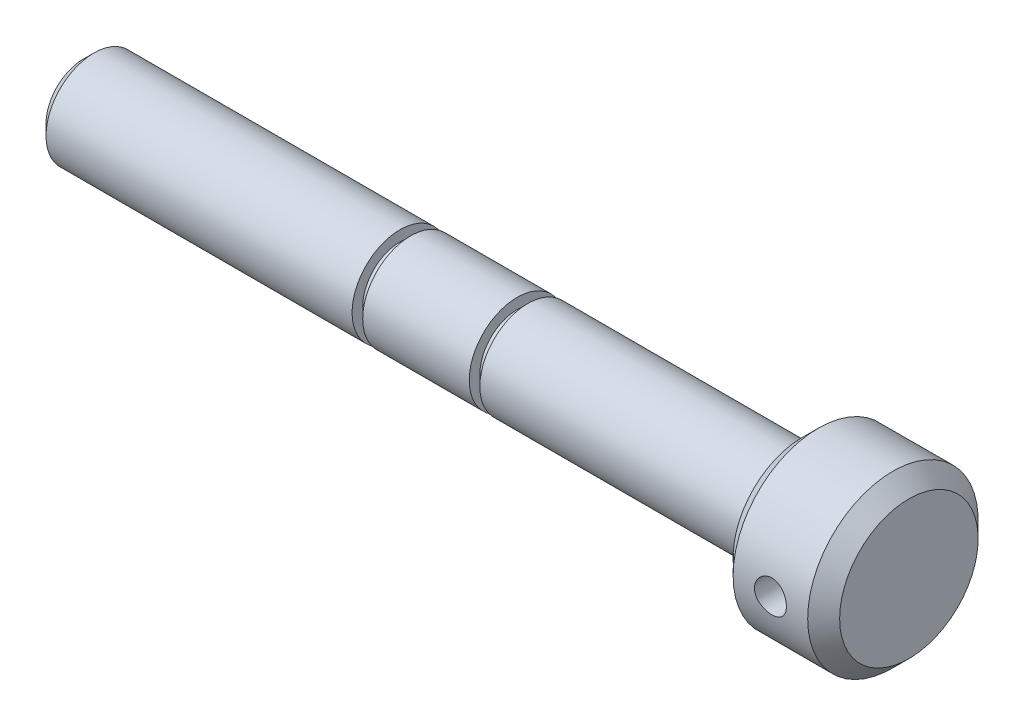
ISO-10303-21;
HEADER;
FILE_DESCRIPTION(('STEP AP214'),'2;1');
FILE_NAME('part.step','',(''),(''),'','','');
FILE_SCHEMA(('AUTOMOTIVE_DESIGN { 1 0 10303 214 1 1 1 1 }'));
ENDSEC;
DATA;
#1=APPLICATION_CONTEXT('core data for automotive mechanical design processes');
#2=APPLICATION_PROTOCOL_DEFINITION('international standard','automotive_design',2000,#1);
#3=PRODUCT_CONTEXT('',#1,'mechanical');
#4=PRODUCT('Part','Part','',(#3));
#5=PRODUCT_RELATED_PRODUCT_CATEGORY('part','',(#4));
#6=PRODUCT_DEFINITION_FORMATION('','',#4);
#7=PRODUCT_DEFINITION_CONTEXT('part definition',#1,'design');
#8=PRODUCT_DEFINITION('design','',#6,#7);
#9=PRODUCT_DEFINITION_SHAPE('','',#8);
#10=(LENGTH_UNIT() NAMED_UNIT(*) SI_UNIT(.MILLI.,.METRE.));
#11=(NAMED_UNIT(*) PLANE_ANGLE_UNIT() SI_UNIT($,.RADIAN.));
#12=(NAMED_UNIT(*) SI_UNIT($,.STERADIAN.) SOLID_ANGLE_UNIT());
#13=UNCERTAINTY_MEASURE_WITH_UNIT(LENGTH_MEASURE(1.E-05),#10,'distance_accuracy_value','');
#14=(GEOMETRIC_REPRESENTATION_CONTEXT(3) GLOBAL_UNCERTAINTY_ASSIGNED_CONTEXT((#13)) GLOBAL_UNIT_ASSIGNED_CONTEXT((#10,
#11,#12)) REPRESENTATION_CONTEXT('',''));
#15=CARTESIAN_POINT('',(0.,0.,0.));
#16=DIRECTION('',(0.,0.,1.));
#17=DIRECTION('',(1.,0.,0.));
#18=AXIS2_PLACEMENT_3D('',#15,#16,#17);
#19=CARTESIAN_POINT('',(155.,0.,0.));
#20=DIRECTION('',(-1.,0.,0.));
#21=DIRECTION('',(0.,0.,1.));
#22=AXIS2_PLACEMENT_3D('',#19,#20,#21);
#23=PLANE('',#22);
#24=CARTESIAN_POINT('',(155.,0.,0.));
#25=DIRECTION('',(-1.,0.,0.));
#26=DIRECTION('',(0.,0.,1.));
#27=AXIS2_PLACEMENT_3D('',#24,#25,#26);
#28=CIRCLE('',#27,13.);
#29=CARTESIAN_POINT('',(155.,0.,13.));
#30=VERTEX_POINT('',#29);
#31=EDGE_CURVE('E161',#30,#30,#28,.F.);
#32=ORIENTED_EDGE('',*,*,#31,.T.);
#33=EDGE_LOOP('',(#32));
#34=FACE_BOUND('',#33,.T.);
#35=ADVANCED_FACE('F50',(#34),#23,.F.);
#36=CARTESIAN_POINT('',(0.,0.,0.));
#37=DIRECTION('',(-1.,0.,0.));
#38=DIRECTION('',(0.,0.,1.));
#39=AXIS2_PLACEMENT_3D('',#36,#37,#38);
#40=CYLINDRICAL_SURFACE('',#39,16.);
#41=CARTESIAN_POINT('',(148.,0.,-16.));
#42=CARTESIAN_POINT('',(147.999993620823,0.166943492930943,-15.999996976677));
#43=CARTESIAN_POINT('',(147.986017846761,0.3339699854602,-15.9973601984343));
#44=CARTESIAN_POINT('',(147.930520009763,0.663316259683598,-15.9870957178104));
#45=CARTESIAN_POINT('',(147.888974698721,0.825631948304453,-15.9794638033379));
#46=CARTESIAN_POINT('',(147.779654597481,1.14074592370361,-15.9600627753092));
#47=CARTESIAN_POINT('',(147.711903495095,1.2935526613707,-15.9482973989297));
#48=CARTESIAN_POINT('',(147.552162246154,1.58561594618802,-15.9219142119957));
#49=CARTESIAN_POINT('',(147.46017406171,1.72487358895465,-15.9072966323658));
#50=CARTESIAN_POINT('',(147.253400463993,1.987567431861,-15.8766267286101));
#51=CARTESIAN_POINT('',(147.13838111066,2.11081791006366,-15.860560697127));
#52=CARTESIAN_POINT('',(146.889313381825,2.33639212270738,-15.828906369173));
#53=CARTESIAN_POINT('',(146.755263640461,2.43871435378482,-15.8133181070905));
#54=CARTESIAN_POINT('',(146.470627823272,2.62029997331585,-15.7842510249001));
#55=CARTESIAN_POINT('',(146.319919259366,2.6993744393921,-15.7707898777236));
#56=CARTESIAN_POINT('',(146.007062169646,2.83101048664565,-15.7476942642397));
#57=CARTESIAN_POINT('',(145.844914631778,2.88357435426196,-15.7380594679392));
#58=CARTESIAN_POINT('',(145.515769538171,2.96010107007,-15.723845391491));
#59=CARTESIAN_POINT('',(145.348849805593,2.98438780384077,-15.7192089073281));
#60=CARTESIAN_POINT('',(145.013245230383,3.00467616190692,-15.7153439430552));
#61=CARTESIAN_POINT('',(144.844560547395,3.00068032270747,-15.7161149779752));
#62=CARTESIAN_POINT('',(144.512560949468,2.96477959204724,-15.7229258540351));
#63=CARTESIAN_POINT('',(144.3492045714,2.93324299992089,-15.7288961629467));
#64=CARTESIAN_POINT('',(144.030143160435,2.84373598792413,-15.7453236656933));
#65=CARTESIAN_POINT('',(143.874438452981,2.78576444478997,-15.7557810501903));
#66=CARTESIAN_POINT('',(143.574022641999,2.64467294358598,-15.7800771058518));
#67=CARTESIAN_POINT('',(143.429383058838,2.5614042706491,-15.7939356764673));
#68=CARTESIAN_POINT('',(143.15599054292,2.37218737860831,-15.8234594320584));
#69=CARTESIAN_POINT('',(143.02723922457,2.26623685778531,-15.8391248003104));
#70=CARTESIAN_POINT('',(142.787150088655,2.03267811370594,-15.8708000254433));
#71=CARTESIAN_POINT('',(142.676118695097,1.90475487372135,-15.8868114204806));
#72=CARTESIAN_POINT('',(142.477045518649,1.63193607419765,-15.9171477221664));
#73=CARTESIAN_POINT('',(142.389003966259,1.48704034451154,-15.9314726119049));
#74=CARTESIAN_POINT('',(142.23836449226,1.18406997774934,-15.9568507935502));
#75=CARTESIAN_POINT('',(142.175798441764,1.02597912889299,-15.9678999827258));
#76=CARTESIAN_POINT('',(142.078195813816,0.701278230797388,-15.9854501080544));
#77=CARTESIAN_POINT('',(142.043156311909,0.534669088555567,-15.9919515273599));
#78=CARTESIAN_POINT('',(142.002027937963,0.200297305806761,-15.9996072128396));
#79=CARTESIAN_POINT('',(141.995519216941,0.0325880252682617,-16.0008390182456));
#80=CARTESIAN_POINT('',(142.010510959095,-0.301522496184375,-15.9980308719646));
#81=CARTESIAN_POINT('',(142.03201004613,-0.467923800960776,-15.9939911792886));
#82=CARTESIAN_POINT('',(142.102058070367,-0.793363146436439,-15.9811422300081));
#83=CARTESIAN_POINT('',(142.150394565076,-0.952448522092132,-15.9723704474806));
#84=CARTESIAN_POINT('',(142.272515413558,-1.26025726364927,-15.95103684425));
#85=CARTESIAN_POINT('',(142.346301495132,-1.40897992519021,-15.9384747662267));
#86=CARTESIAN_POINT('',(142.518156256319,-1.69363334302643,-15.9107606071533));
#87=CARTESIAN_POINT('',(142.616481477074,-1.82940655403025,-15.8955817234913));
#88=CARTESIAN_POINT('',(142.834276274725,-2.0826766465291,-15.8643868697942));
#89=CARTESIAN_POINT('',(142.953747826003,-2.20017181952174,-15.8483708216937));
#90=CARTESIAN_POINT('',(143.212344637823,-2.41514591744096,-15.817049513949));
#91=CARTESIAN_POINT('',(143.351709816251,-2.51233832437154,-15.8017565172051));
#92=CARTESIAN_POINT('',(143.645035249048,-2.68193350115574,-15.7738597115706));
#93=CARTESIAN_POINT('',(143.798994960741,-2.75433719227848,-15.761255802747));
#94=CARTESIAN_POINT('',(144.116411734485,-2.87189347025646,-15.7402604841915));
#95=CARTESIAN_POINT('',(144.279818759119,-2.91717737589572,-15.7318488087376));
#96=CARTESIAN_POINT('',(144.612094445043,-2.9796135865247,-15.7201440760483));
#97=CARTESIAN_POINT('',(144.780962487941,-2.99676906541416,-15.7168504413158));
#98=CARTESIAN_POINT('',(145.116496662883,-3.00235524296709,-15.7157839960771));
#99=CARTESIAN_POINT('',(145.283155161914,-2.99123790006997,-15.7179243194859));
#100=CARTESIAN_POINT('',(145.612182844091,-2.94158350757605,-15.7272920132));
#101=CARTESIAN_POINT('',(145.774552052855,-2.90304662178663,-15.7345193531149));
#102=CARTESIAN_POINT('',(146.090148969591,-2.79983775166526,-15.7532101604636));
#103=CARTESIAN_POINT('',(146.243393182692,-2.73521470794505,-15.7646656918993));
#104=CARTESIAN_POINT('',(146.536936508482,-2.58171737824409,-15.7905277510368));
#105=CARTESIAN_POINT('',(146.67723470569,-2.49284137896372,-15.8049344872024));
#106=CARTESIAN_POINT('',(146.943167360085,-2.29178974679071,-15.8353453221549));
#107=CARTESIAN_POINT('',(147.068550825134,-2.17928519728607,-15.8513701070609));
#108=CARTESIAN_POINT('',(147.298810324929,-1.93485585348458,-15.8830566783747));
#109=CARTESIAN_POINT('',(147.40368164196,-1.80292660378324,-15.8987183805466));
#110=CARTESIAN_POINT('',(147.590821905254,-1.52196989014375,-15.928079519361));
#111=CARTESIAN_POINT('',(147.672878856981,-1.37279918128104,-15.9417600198112));
#112=CARTESIAN_POINT('',(147.81063527321,-1.06258022730767,-15.9654323876137));
#113=CARTESIAN_POINT('',(147.866359494094,-0.901543303410502,-15.9754277175807));
#114=CARTESIAN_POINT('',(147.938554628837,-0.616694405650312,-15.9885658141526));
#115=CARTESIAN_POINT('',(147.961557260626,-0.494547620503743,-15.9928294175641));
#116=CARTESIAN_POINT('',(147.992282124233,-0.248282494230316,-15.9985475990802));
#117=CARTESIAN_POINT('',(148.000004744512,-0.124164203305419,-16.0000022485961));
#118=CARTESIAN_POINT('',(148.,0.,-16.));
#119=B_SPLINE_CURVE_WITH_KNOTS('',3,(#41,#42,#43,#44,#45,#46,#47,#48,#49,#50,#51,#52,#53,#54,
#55,#56,#57,#58,#59,#60,#61,#62,#63,#64,#65,#66,#67,#68,#69,#70,#71,#72,#73,#74,#75,#76,#77,#78,
#79,#80,#81,#82,#83,#84,#85,#86,#87,#88,#89,#90,#91,#92,#93,#94,#95,#96,#97,#98,#99,#100,#101,
#102,#103,#104,#105,#106,#107,#108,#109,#110,#111,#112,#113,#114,#115,#116,#117,#118),
.UNSPECIFIED.,.T.,.F.,(4,2,2,2,2,2,2,2,2,2,2,2,2,2,2,2,2,2,2,2,2,2,2,2,2,2,2,2,2,2,2,2,2,2,2,2,
2,2,4),(0.,0.500376401929855,1.0011752850709,1.50152254246182,2.00182930673783,2.5075023602726,
3.01321172567232,3.52292381008715,4.03259192623896,4.53636302890669,5.04008895174511,
5.53718001225533,6.03429219693572,6.5343852525906,7.03452908099719,7.54255536928152,
8.05058675089894,8.55925176643395,9.0678627334749,9.56896348152192,10.0700396092917,
10.5672046781565,11.0644035067606,11.5670355603542,12.069714568262,12.579068739746,
13.0884039790989,13.5952525563712,14.1020439389302,14.6007850446349,15.0995231708301,
15.5973299241538,16.0951718531084,16.6004673993276,17.1058790252451,17.6158409783262,
18.1253225386234,18.4974868904881,18.8696417807908),.UNSPECIFIED.);
#120=CARTESIAN_POINT('',(148.,0.,-16.));
#121=VERTEX_POINT('',#120);
#122=EDGE_CURVE('E10',#121,#121,#119,.T.);
#123=ORIENTED_EDGE('',*,*,#122,.T.);
#124=EDGE_LOOP('',(#123));
#125=FACE_BOUND('',#124,.T.);
#126=CARTESIAN_POINT('',(148.,0.,16.));
#127=CARTESIAN_POINT('',(147.999993620823,-0.166943492930943,15.999996976677));
#128=CARTESIAN_POINT('',(147.986017846761,-0.3339699854602,15.9973601984343));
#129=CARTESIAN_POINT('',(147.930520009763,-0.663316259683598,15.9870957178104));
#130=CARTESIAN_POINT('',(147.888974698721,-0.825631948304453,15.9794638033379));
#131=CARTESIAN_POINT('',(147.779654597481,-1.14074592370361,15.9600627753092));
#132=CARTESIAN_POINT('',(147.711903495095,-1.2935526613707,15.9482973989297));
#133=CARTESIAN_POINT('',(147.552162246154,-1.58561594618802,15.9219142119957));
#134=CARTESIAN_POINT('',(147.46017406171,-1.72487358895465,15.9072966323658));
#135=CARTESIAN_POINT('',(147.253400463993,-1.987567431861,15.8766267286101));
#136=CARTESIAN_POINT('',(147.13838111066,-2.11081791006366,15.860560697127));
#137=CARTESIAN_POINT('',(146.889313381825,-2.33639212270738,15.828906369173));
#138=CARTESIAN_POINT('',(146.755263640461,-2.43871435378482,15.8133181070905));
#139=CARTESIAN_POINT('',(146.470627823272,-2.62029997331585,15.7842510249001));
#140=CARTESIAN_POINT('',(146.319919259366,-2.6993744393921,15.7707898777236));
#141=CARTESIAN_POINT('',(146.007062169646,-2.83101048664565,15.7476942642397));
#142=CARTESIAN_POINT('',(145.844914631778,-2.88357435426196,15.7380594679392));
#143=CARTESIAN_POINT('',(145.515769538171,-2.96010107007,15.723845391491));
#144=CARTESIAN_POINT('',(145.348849805593,-2.98438780384077,15.7192089073281));
#145=CARTESIAN_POINT('',(145.013245230383,-3.00467616190692,15.7153439430552));
#146=CARTESIAN_POINT('',(144.844560547395,-3.00068032270747,15.7161149779752));
#147=CARTESIAN_POINT('',(144.512560949468,-2.96477959204724,15.7229258540351));
#148=CARTESIAN_POINT('',(144.3492045714,-2.93324299992089,15.7288961629467));
#149=CARTESIAN_POINT('',(144.030143160435,-2.84373598792413,15.7453236656933));
#150=CARTESIAN_POINT('',(143.874438452981,-2.78576444478997,15.7557810501903));
#151=CARTESIAN_POINT('',(143.574022641999,-2.64467294358598,15.7800771058518));
#152=CARTESIAN_POINT('',(143.429383058838,-2.5614042706491,15.7939356764673));
#153=CARTESIAN_POINT('',(143.15599054292,-2.37218737860831,15.8234594320584));
#154=CARTESIAN_POINT('',(143.02723922457,-2.26623685778531,15.8391248003104));
#155=CARTESIAN_POINT('',(142.787150088655,-2.03267811370594,15.8708000254433));
#156=CARTESIAN_POINT('',(142.676118695097,-1.90475487372135,15.8868114204806));
#157=CARTESIAN_POINT('',(142.477045518649,-1.63193607419765,15.9171477221664));
#158=CARTESIAN_POINT('',(142.389003966259,-1.48704034451154,15.9314726119049));
#159=CARTESIAN_POINT('',(142.23836449226,-1.18406997774934,15.9568507935502));
#160=CARTESIAN_POINT('',(142.175798441764,-1.02597912889299,15.9678999827258));
#161=CARTESIAN_POINT('',(142.078195813816,-0.701278230797388,15.9854501080544));
#162=CARTESIAN_POINT('',(142.043156311909,-0.534669088555567,15.9919515273599));
#163=CARTESIAN_POINT('',(142.002027937963,-0.200297305806761,15.9996072128396));
#164=CARTESIAN_POINT('',(141.995519216941,-0.0325880252682617,16.0008390182456));
#165=CARTESIAN_POINT('',(142.010510959095,0.301522496184375,15.9980308719646));
#166=CARTESIAN_POINT('',(142.03201004613,0.467923800960776,15.9939911792886));
#167=CARTESIAN_POINT('',(142.102058070367,0.793363146436439,15.9811422300081));
#168=CARTESIAN_POINT('',(142.150394565076,0.952448522092132,15.9723704474806));
#169=CARTESIAN_POINT('',(142.272515413558,1.26025726364927,15.95103684425));
#170=CARTESIAN_POINT('',(142.346301495132,1.40897992519021,15.9384747662267));
#171=CARTESIAN_POINT('',(142.518156256319,1.69363334302643,15.9107606071533));
#172=CARTESIAN_POINT('',(142.616481477074,1.82940655403025,15.8955817234913));
#173=CARTESIAN_POINT('',(142.834276274725,2.0826766465291,15.8643868697942));
#174=CARTESIAN_POINT('',(142.953747826003,2.20017181952174,15.8483708216937));
#175=CARTESIAN_POINT('',(143.212344637823,2.41514591744096,15.817049513949));
#176=CARTESIAN_POINT('',(143.351709816251,2.51233832437154,15.8017565172051));
#177=CARTESIAN_POINT('',(143.645035249048,2.68193350115574,15.7738597115706));
#178=CARTESIAN_POINT('',(143.798994960741,2.75433719227848,15.761255802747));
#179=CARTESIAN_POINT('',(144.116411734485,2.87189347025646,15.7402604841915));
#180=CARTESIAN_POINT('',(144.279818759119,2.91717737589572,15.7318488087376));
#181=CARTESIAN_POINT('',(144.612094445043,2.9796135865247,15.7201440760483));
#182=CARTESIAN_POINT('',(144.780962487941,2.99676906541416,15.7168504413158));
#183=CARTESIAN_POINT('',(145.116496662883,3.00235524296709,15.7157839960771));
#184=CARTESIAN_POINT('',(145.283155161914,2.99123790006997,15.7179243194859));
#185=CARTESIAN_POINT('',(145.612182844091,2.94158350757605,15.7272920132));
#186=CARTESIAN_POINT('',(145.774552052855,2.90304662178663,15.7345193531149));
#187=CARTESIAN_POINT('',(146.090148969591,2.79983775166526,15.7532101604636));
#188=CARTESIAN_POINT('',(146.243393182692,2.73521470794505,15.7646656918993));
#189=CARTESIAN_POINT('',(146.536936508482,2.58171737824409,15.7905277510368));
#190=CARTESIAN_POINT('',(146.67723470569,2.49284137896372,15.8049344872024));
#191=CARTESIAN_POINT('',(146.943167360085,2.29178974679071,15.8353453221549));
#192=CARTESIAN_POINT('',(147.068550825134,2.17928519728607,15.8513701070609));
#193=CARTESIAN_POINT('',(147.298810324929,1.93485585348458,15.8830566783747));
#194=CARTESIAN_POINT('',(147.40368164196,1.80292660378324,15.8987183805466));
#195=CARTESIAN_POINT('',(147.590821905254,1.52196989014375,15.928079519361));
#196=CARTESIAN_POINT('',(147.672878856981,1.37279918128104,15.9417600198112));
#197=CARTESIAN_POINT('',(147.81063527321,1.06258022730767,15.9654323876137));
#198=CARTESIAN_POINT('',(147.866359494094,0.901543303410502,15.9754277175807));
#199=CARTESIAN_POINT('',(147.938554628837,0.616694405650312,15.9885658141526));
#200=CARTESIAN_POINT('',(147.961557260626,0.494547620503743,15.9928294175641));
#201=CARTESIAN_POINT('',(147.992282124233,0.248282494230316,15.9985475990802));
#202=CARTESIAN_POINT('',(148.000004744512,0.124164203305419,16.0000022485961));
#203=CARTESIAN_POINT('',(148.,0.,16.));
#204=B_SPLINE_CURVE_WITH_KNOTS('',3,(#126,#127,#128,#129,#130,#131,#132,#133,#134,#135,#136,
#137,#138,#139,#140,#141,#142,#143,#144,#145,#146,#147,#148,#149,#150,#151,#152,#153,#154,#155,
#156,#157,#158,#159,#160,#161,#162,#163,#164,#165,#166,#167,#168,#169,#170,#171,#172,#173,#174,
#175,#176,#177,#178,#179,#180,#181,#182,#183,#184,#185,#186,#187,#188,#189,#190,#191,#192,#193,
#194,#195,#196,#197,#198,#199,#200,#201,#202,#203),.UNSPECIFIED.,.T.,.F.,(4,2,2,2,2,2,2,2,2,2,2,
2,2,2,2,2,2,2,2,2,2,2,2,2,2,2,2,2,2,2,2,2,2,2,2,2,2,2,4),(0.,0.500376401929855,1.0011752850709,
1.50152254246182,2.00182930673783,2.5075023602726,3.01321172567232,3.52292381008715,
4.03259192623896,4.53636302890669,5.04008895174511,5.53718001225533,6.03429219693572,
6.5343852525906,7.03452908099719,7.54255536928152,8.05058675089894,8.55925176643395,
9.0678627334749,9.56896348152192,10.0700396092917,10.5672046781565,11.0644035067606,
11.5670355603542,12.069714568262,12.579068739746,13.0884039790989,13.5952525563712,
14.1020439389302,14.6007850446349,15.0995231708301,15.5973299241538,16.0951718531084,
16.6004673993276,17.1058790252451,17.6158409783262,18.1253225386234,18.4974868904881,
18.8696417807908),.UNSPECIFIED.);
#205=CARTESIAN_POINT('',(148.,0.,16.));
#206=VERTEX_POINT('',#205);
#207=EDGE_CURVE('E58',#206,#206,#204,.T.);
#208=ORIENTED_EDGE('',*,*,#207,.T.);
#209=EDGE_LOOP('',(#208));
#210=FACE_BOUND('',#209,.T.);
#211=CARTESIAN_POINT('',(152.,0.,0.));
#212=DIRECTION('',(-1.,0.,0.));
#213=DIRECTION('',(0.,0.,1.));
#214=AXIS2_PLACEMENT_3D('',#211,#212,#213);
#215=CIRCLE('',#214,16.);
#216=CARTESIAN_POINT('',(152.,0.,16.));
#217=VERTEX_POINT('',#216);
#218=EDGE_CURVE('E163',#217,#217,#215,.T.);
#219=ORIENTED_EDGE('',*,*,#218,.T.);
#220=EDGE_LOOP('',(#219));
#221=FACE_BOUND('',#220,.T.);
#222=CARTESIAN_POINT('',(138.,0.,0.));
#223=DIRECTION('',(1.,0.,0.));
#224=DIRECTION('',(0.,0.,-1.));
#225=AXIS2_PLACEMENT_3D('',#222,#223,#224);
#226=CIRCLE('',#225,16.);
#227=CARTESIAN_POINT('',(138.,0.,-16.));
#228=VERTEX_POINT('',#227);
#229=EDGE_CURVE('E158',#228,#228,#226,.T.);
#230=ORIENTED_EDGE('',*,*,#229,.T.);
#231=EDGE_LOOP('',(#230));
#232=FACE_BOUND('',#231,.T.);
#233=ADVANCED_FACE('F74',(#125,#210,#221,#232),#40,.T.);
#234=CARTESIAN_POINT('',(135.,16.,0.));
#235=DIRECTION('',(1.,0.,0.));
#236=DIRECTION('',(0.,0.,-1.));
#237=AXIS2_PLACEMENT_3D('',#234,#235,#236);
#238=PLANE('',#237);
#239=CARTESIAN_POINT('',(135.,0.,0.));
#240=DIRECTION('',(1.,0.,0.));
#241=DIRECTION('',(0.,0.,-1.));
#242=AXIS2_PLACEMENT_3D('',#239,#240,#241);
#243=CIRCLE('',#242,12.9999999999999);
#244=CARTESIAN_POINT('',(135.,0.,-12.9999999999999));
#245=VERTEX_POINT('',#244);
#246=EDGE_CURVE('E159',#245,#245,#243,.F.);
#247=ORIENTED_EDGE('',*,*,#246,.T.);
#248=EDGE_LOOP('',(#247));
#249=FACE_BOUND('',#248,.T.);
#250=CARTESIAN_POINT('',(135.,0.,0.));
#251=DIRECTION('',(-1.,0.,0.));
#252=DIRECTION('',(0.,0.,1.));
#253=AXIS2_PLACEMENT_3D('',#250,#251,#252);
#254=CIRCLE('',#253,9.00000000000002);
#255=CARTESIAN_POINT('',(135.,0.,9.00000000000002));
#256=VERTEX_POINT('',#255);
#257=EDGE_CURVE('E168',#256,#256,#254,.T.);
#258=ORIENTED_EDGE('',*,*,#257,.F.);
#259=EDGE_LOOP('',(#258));
#260=FACE_BOUND('',#259,.T.);
#261=ADVANCED_FACE('F122',(#249,#260),#238,.F.);
#262=CARTESIAN_POINT('',(0.,0.,0.));
#263=DIRECTION('',(-1.,0.,0.));
#264=DIRECTION('',(0.,0.,1.));
#265=AXIS2_PLACEMENT_3D('',#262,#263,#264);
#266=CYLINDRICAL_SURFACE('',#265,9.00000000000001);
#267=CARTESIAN_POINT('',(83.46,0.,0.));
#268=DIRECTION('',(-1.,0.,0.));
#269=DIRECTION('',(0.,0.,1.));
#270=AXIS2_PLACEMENT_3D('',#267,#268,#269);
#271=CIRCLE('',#270,9.00000000000001);
#272=CARTESIAN_POINT('',(83.46,0.,9.00000000000001));
#273=VERTEX_POINT('',#272);
#274=EDGE_CURVE('E174',#273,#273,#271,.T.);
#275=ORIENTED_EDGE('',*,*,#274,.F.);
#276=EDGE_LOOP('',(#275));
#277=FACE_BOUND('',#276,.T.);
#278=ORIENTED_EDGE('',*,*,#257,.T.);
#279=EDGE_LOOP('',(#278));
#280=FACE_BOUND('',#279,.T.);
#281=ADVANCED_FACE('F120',(#277,#280),#266,.T.);
#282=CARTESIAN_POINT('',(83.46,9.00000000000001,0.));
#283=DIRECTION('',(1.,0.,0.));
#284=DIRECTION('',(0.,0.,-1.));
#285=AXIS2_PLACEMENT_3D('',#282,#283,#284);
#286=PLANE('',#285);
#287=CARTESIAN_POINT('',(83.46,0.,0.));
#288=DIRECTION('',(-1.,0.,0.));
#289=DIRECTION('',(0.,0.,1.));
#290=AXIS2_PLACEMENT_3D('',#287,#288,#289);
#291=CIRCLE('',#290,7.);
#292=CARTESIAN_POINT('',(83.46,0.,7.));
#293=VERTEX_POINT('',#292);
#294=EDGE_CURVE('E176',#293,#293,#291,.T.);
#295=ORIENTED_EDGE('',*,*,#294,.F.);
#296=EDGE_LOOP('',(#295));
#297=FACE_BOUND('',#296,.T.);
#298=ORIENTED_EDGE('',*,*,#274,.T.);
#299=EDGE_LOOP('',(#298));
#300=FACE_BOUND('',#299,.T.);
#301=ADVANCED_FACE('F116',(#297,#300),#286,.F.);
#302=CARTESIAN_POINT('',(0.,0.,0.));
#303=DIRECTION('',(-1.,0.,0.));
#304=DIRECTION('',(0.,0.,1.));
#305=AXIS2_PLACEMENT_3D('',#302,#303,#304);
#306=CYLINDRICAL_SURFACE('',#305,7.);
#307=CARTESIAN_POINT('',(81.46,0.,0.));
#308=DIRECTION('',(-1.,0.,0.));
#309=DIRECTION('',(0.,0.,1.));
#310=AXIS2_PLACEMENT_3D('',#307,#308,#309);
#311=CIRCLE('',#310,7.);
#312=CARTESIAN_POINT('',(81.46,0.,7.));
#313=VERTEX_POINT('',#312);
#314=EDGE_CURVE('E178',#313,#313,#311,.T.);
#315=ORIENTED_EDGE('',*,*,#314,.F.);
#316=EDGE_LOOP('',(#315));
#317=FACE_BOUND('',#316,.T.);
#318=ORIENTED_EDGE('',*,*,#294,.T.);
#319=EDGE_LOOP('',(#318));
#320=FACE_BOUND('',#319,.T.);
#321=ADVANCED_FACE('F115',(#317,#320),#306,.T.);
#322=CARTESIAN_POINT('',(81.46,7.,0.));
#323=DIRECTION('',(-1.,0.,0.));
#324=DIRECTION('',(0.,0.,1.));
#325=AXIS2_PLACEMENT_3D('',#322,#323,#324);
#326=PLANE('',#325);
#327=CARTESIAN_POINT('',(81.46,0.,0.));
#328=DIRECTION('',(-1.,0.,0.));
#329=DIRECTION('',(0.,0.,1.));
#330=AXIS2_PLACEMENT_3D('',#327,#328,#329);
#331=CIRCLE('',#330,9.00000000000001);
#332=CARTESIAN_POINT('',(81.46,0.,9.00000000000001));
#333=VERTEX_POINT('',#332);
#334=EDGE_CURVE('E185',#333,#333,#331,.T.);
#335=ORIENTED_EDGE('',*,*,#334,.F.);
#336=EDGE_LOOP('',(#335));
#337=FACE_BOUND('',#336,.T.);
#338=ORIENTED_EDGE('',*,*,#314,.T.);
#339=EDGE_LOOP('',(#338));
#340=FACE_BOUND('',#339,.T.);
#341=ADVANCED_FACE('F107',(#337,#340),#326,.F.);
#342=CARTESIAN_POINT('',(0.,0.,0.));
#343=DIRECTION('',(-1.,0.,0.));
#344=DIRECTION('',(0.,0.,1.));
#345=AXIS2_PLACEMENT_3D('',#342,#343,#344);
#346=CYLINDRICAL_SURFACE('',#345,9.00000000000001);
#347=CARTESIAN_POINT('',(61.46,0.,0.));
#348=DIRECTION('',(-1.,0.,0.));
#349=DIRECTION('',(0.,0.,1.));
#350=AXIS2_PLACEMENT_3D('',#347,#348,#349);
#351=CIRCLE('',#350,9.00000000000001);
#352=CARTESIAN_POINT('',(61.46,0.,9.00000000000001));
#353=VERTEX_POINT('',#352);
#354=EDGE_CURVE('E183',#353,#353,#351,.T.);
#355=ORIENTED_EDGE('',*,*,#354,.F.);
#356=EDGE_LOOP('',(#355));
#357=FACE_BOUND('',#356,.T.);
#358=ORIENTED_EDGE('',*,*,#334,.T.);
#359=EDGE_LOOP('',(#358));
#360=FACE_BOUND('',#359,.T.);
#361=ADVANCED_FACE('F102',(#357,#360),#346,.T.);
#362=CARTESIAN_POINT('',(61.46,9.00000000000001,0.));
#363=DIRECTION('',(1.,0.,0.));
#364=DIRECTION('',(0.,0.,-1.));
#365=AXIS2_PLACEMENT_3D('',#362,#363,#364);
#366=PLANE('',#365);
#367=CARTESIAN_POINT('',(61.46,0.,0.));
#368=DIRECTION('',(-1.,0.,0.));
#369=DIRECTION('',(0.,0.,1.));
#370=AXIS2_PLACEMENT_3D('',#367,#368,#369);
#371=CIRCLE('',#370,7.);
#372=CARTESIAN_POINT('',(61.46,0.,7.));
#373=VERTEX_POINT('',#372);
#374=EDGE_CURVE('E189',#373,#373,#371,.T.);
#375=ORIENTED_EDGE('',*,*,#374,.F.);
#376=EDGE_LOOP('',(#375));
#377=FACE_BOUND('',#376,.T.);
#378=ORIENTED_EDGE('',*,*,#354,.T.);
#379=EDGE_LOOP('',(#378));
#380=FACE_BOUND('',#379,.T.);
#381=ADVANCED_FACE('F99',(#377,#380),#366,.F.);
#382=CARTESIAN_POINT('',(0.,0.,0.));
#383=DIRECTION('',(-1.,0.,0.));
#384=DIRECTION('',(0.,0.,1.));
#385=AXIS2_PLACEMENT_3D('',#382,#383,#384);
#386=CYLINDRICAL_SURFACE('',#385,7.);
#387=CARTESIAN_POINT('',(59.46,0.,0.));
#388=DIRECTION('',(-1.,0.,0.));
#389=DIRECTION('',(0.,0.,1.));
#390=AXIS2_PLACEMENT_3D('',#387,#388,#389);
#391=CIRCLE('',#390,7.);
#392=CARTESIAN_POINT('',(59.46,0.,7.));
#393=VERTEX_POINT('',#392);
#394=EDGE_CURVE('E191',#393,#393,#391,.T.);
#395=ORIENTED_EDGE('',*,*,#394,.F.);
#396=EDGE_LOOP('',(#395));
#397=FACE_BOUND('',#396,.T.);
#398=ORIENTED_EDGE('',*,*,#374,.T.);
#399=EDGE_LOOP('',(#398));
#400=FACE_BOUND('',#399,.T.);
#401=ADVANCED_FACE('F96',(#397,#400),#386,.T.);
#402=CARTESIAN_POINT('',(59.46,7.,0.));
#403=DIRECTION('',(-1.,0.,0.));
#404=DIRECTION('',(0.,0.,1.));
#405=AXIS2_PLACEMENT_3D('',#402,#403,#404);
#406=PLANE('',#405);
#407=CARTESIAN_POINT('',(59.46,0.,0.));
#408=DIRECTION('',(-1.,0.,0.));
#409=DIRECTION('',(0.,0.,1.));
#410=AXIS2_PLACEMENT_3D('',#407,#408,#409);
#411=CIRCLE('',#410,9.00000000000001);
#412=CARTESIAN_POINT('',(59.46,0.,9.00000000000001));
#413=VERTEX_POINT('',#412);
#414=EDGE_CURVE('E193',#413,#413,#411,.T.);
#415=ORIENTED_EDGE('',*,*,#414,.F.);
#416=EDGE_LOOP('',(#415));
#417=FACE_BOUND('',#416,.T.);
#418=ORIENTED_EDGE('',*,*,#394,.T.);
#419=EDGE_LOOP('',(#418));
#420=FACE_BOUND('',#419,.T.);
#421=ADVANCED_FACE('F95',(#417,#420),#406,.F.);
#422=CARTESIAN_POINT('',(0.,0.,0.));
#423=DIRECTION('',(-1.,0.,0.));
#424=DIRECTION('',(0.,0.,1.));
#425=AXIS2_PLACEMENT_3D('',#422,#423,#424);
#426=CYLINDRICAL_SURFACE('',#425,9.);
#427=CARTESIAN_POINT('',(1.99999999999999,0.,0.));
#428=DIRECTION('',(1.,0.,0.));
#429=DIRECTION('',(0.,0.,-1.));
#430=AXIS2_PLACEMENT_3D('',#427,#428,#429);
#431=CIRCLE('',#430,9.);
#432=CARTESIAN_POINT('',(1.99999999999999,0.,-9.));
#433=VERTEX_POINT('',#432);
#434=EDGE_CURVE('E63',#433,#433,#431,.T.);
#435=ORIENTED_EDGE('',*,*,#434,.T.);
#436=EDGE_LOOP('',(#435));
#437=FACE_BOUND('',#436,.T.);
#438=ORIENTED_EDGE('',*,*,#414,.T.);
#439=EDGE_LOOP('',(#438));
#440=FACE_BOUND('',#439,.T.);
#441=ADVANCED_FACE('F86',(#437,#440),#426,.T.);
#442=CARTESIAN_POINT('',(0.,9.,0.));
#443=DIRECTION('',(1.,0.,0.));
#444=DIRECTION('',(0.,0.,-1.));
#445=AXIS2_PLACEMENT_3D('',#442,#443,#444);
#446=PLANE('',#445);
#447=CARTESIAN_POINT('',(0.,0.,0.));
#448=DIRECTION('',(1.,0.,0.));
#449=DIRECTION('',(0.,0.,-1.));
#450=AXIS2_PLACEMENT_3D('',#447,#448,#449);
#451=CIRCLE('',#450,7.00000000000003);
#452=CARTESIAN_POINT('',(0.,0.,-7.00000000000003));
#453=VERTEX_POINT('',#452);
#454=EDGE_CURVE('E67',#453,#453,#451,.F.);
#455=ORIENTED_EDGE('',*,*,#454,.T.);
#456=EDGE_LOOP('',(#455));
#457=FACE_BOUND('',#456,.T.);
#458=ADVANCED_FACE('F82',(#457),#446,.F.);
#459=CARTESIAN_POINT('',(152.,0.,0.));
#460=DIRECTION('',(-1.,0.,0.));
#461=DIRECTION('',(0.,0.,1.));
#462=AXIS2_PLACEMENT_3D('',#459,#460,#461);
#463=CONICAL_SURFACE('',#462,16.,0.785398163397445);
#464=CARTESIAN_POINT('',(155.,0.,13.));
#465=CARTESIAN_POINT('',(154.96875,0.,13.03125));
#466=CARTESIAN_POINT('',(154.9375,0.,13.0625));
#467=CARTESIAN_POINT('',(154.875,0.,13.125));
#468=CARTESIAN_POINT('',(154.84375,0.,13.15625));
#469=CARTESIAN_POINT('',(154.78125,0.,13.21875));
#470=CARTESIAN_POINT('',(154.75,0.,13.25));
#471=CARTESIAN_POINT('',(154.6875,0.,13.3125));
#472=CARTESIAN_POINT('',(154.65625,0.,13.34375));
#473=CARTESIAN_POINT('',(154.59375,0.,13.40625));
#474=CARTESIAN_POINT('',(154.5625,0.,13.4375));
#475=CARTESIAN_POINT('',(154.5,0.,13.5));
#476=CARTESIAN_POINT('',(154.46875,0.,13.53125));
#477=CARTESIAN_POINT('',(154.40625,0.,13.59375));
#478=CARTESIAN_POINT('',(154.375,0.,13.625));
#479=CARTESIAN_POINT('',(154.3125,0.,13.6875));
#480=CARTESIAN_POINT('',(154.28125,0.,13.71875));
#481=CARTESIAN_POINT('',(154.21875,0.,13.78125));
#482=CARTESIAN_POINT('',(154.1875,0.,13.8125));
#483=CARTESIAN_POINT('',(154.125,0.,13.875));
#484=CARTESIAN_POINT('',(154.09375,0.,13.90625));
#485=CARTESIAN_POINT('',(154.03125,0.,13.96875));
#486=CARTESIAN_POINT('',(154.,0.,14.));
#487=CARTESIAN_POINT('',(153.9375,0.,14.0625));
#488=CARTESIAN_POINT('',(153.90625,0.,14.09375));
#489=CARTESIAN_POINT('',(153.84375,0.,14.15625));
#490=CARTESIAN_POINT('',(153.8125,0.,14.1875));
#491=CARTESIAN_POINT('',(153.75,0.,14.25));
#492=CARTESIAN_POINT('',(153.71875,0.,14.28125));
#493=CARTESIAN_POINT('',(153.65625,0.,14.34375));
#494=CARTESIAN_POINT('',(153.625,0.,14.375));
#495=CARTESIAN_POINT('',(153.5625,0.,14.4375));
#496=CARTESIAN_POINT('',(153.53125,0.,14.46875));
#497=CARTESIAN_POINT('',(153.46875,0.,14.53125));
#498=CARTESIAN_POINT('',(153.4375,0.,14.5625));
#499=CARTESIAN_POINT('',(153.375,0.,14.625));
#500=CARTESIAN_POINT('',(153.34375,0.,14.65625));
#501=CARTESIAN_POINT('',(153.28125,0.,14.71875));
#502=CARTESIAN_POINT('',(153.25,0.,14.75));
#503=CARTESIAN_POINT('',(153.1875,0.,14.8125));
#504=CARTESIAN_POINT('',(153.15625,0.,14.84375));
#505=CARTESIAN_POINT('',(153.09375,0.,14.90625));
#506=CARTESIAN_POINT('',(153.0625,0.,14.9375));
#507=CARTESIAN_POINT('',(153.,0.,15.));
#508=CARTESIAN_POINT('',(152.96875,0.,15.03125));
#509=CARTESIAN_POINT('',(152.90625,0.,15.09375));
#510=CARTESIAN_POINT('',(152.875,0.,15.125));
#511=CARTESIAN_POINT('',(152.8125,0.,15.1875));
#512=CARTESIAN_POINT('',(152.78125,0.,15.21875));
#513=CARTESIAN_POINT('',(152.71875,0.,15.28125));
#514=CARTESIAN_POINT('',(152.6875,0.,15.3125));
#515=CARTESIAN_POINT('',(152.625,0.,15.375));
#516=CARTESIAN_POINT('',(152.59375,0.,15.40625));
#517=CARTESIAN_POINT('',(152.53125,0.,15.46875));
#518=CARTESIAN_POINT('',(152.5,0.,15.5));
#519=CARTESIAN_POINT('',(152.4375,0.,15.5625));
#520=CARTESIAN_POINT('',(152.40625,0.,15.59375));
#521=CARTESIAN_POINT('',(152.34375,0.,15.65625));
#522=CARTESIAN_POINT('',(152.3125,0.,15.6875));
#523=CARTESIAN_POINT('',(152.25,0.,15.75));
#524=CARTESIAN_POINT('',(152.21875,0.,15.78125));
#525=CARTESIAN_POINT('',(152.15625,0.,15.84375));
#526=CARTESIAN_POINT('',(152.125,0.,15.875));
#527=CARTESIAN_POINT('',(152.0625,0.,15.9375));
#528=CARTESIAN_POINT('',(152.03125,0.,15.96875));
#529=CARTESIAN_POINT('',(152.,0.,16.));
#530=B_SPLINE_CURVE_WITH_KNOTS('',3,(#464,#465,#466,#467,#468,#469,#470,#471,#472,#473,#474,
#475,#476,#477,#478,#479,#480,#481,#482,#483,#484,#485,#486,#487,#488,#489,#490,#491,#492,#493,
#494,#495,#496,#497,#498,#499,#500,#501,#502,#503,#504,#505,#506,#507,#508,#509,#510,#511,#512,
#513,#514,#515,#516,#517,#518,#519,#520,#521,#522,#523,#524,#525,#526,#527,#528,#529),
.UNSPECIFIED.,.F.,.F.,(4,2,2,2,2,2,2,2,2,2,2,2,2,2,2,2,2,2,2,2,2,2,2,2,2,2,2,2,2,2,2,2,4),(0.,
0.132582521472459,0.265165042944938,0.397747564417419,0.530330085889898,0.662912607362377,
0.795495128834856,0.928077650307315,1.0606601717798,1.19324269325227,1.32582521472475,
1.45840773619723,1.59099025766971,1.72357277914217,1.85615530061465,1.98873782208713,
2.12132034355961,2.25390286503209,2.38648538650457,2.51906790797705,2.65165042944951,
2.78423295092198,2.91681547239446,3.04939799386694,3.18198051533942,3.3145630368119,
3.44714555828436,3.57972807975684,3.71231060122932,3.8448931227018,3.97747564417428,
4.11005816564676,4.24264068711924),.UNSPECIFIED.);
#531=EDGE_CURVE('BSEAM87',#30,#217,#530,.T.);
#532=ORIENTED_EDGE('',*,*,#31,.F.);
#533=ORIENTED_EDGE('',*,*,#218,.F.);
#534=ORIENTED_EDGE('',*,*,#531,.T.);
#535=ORIENTED_EDGE('',*,*,#531,.F.);
#536=EDGE_LOOP('',(#532,#534,#533,#535));
#537=FACE_BOUND('',#536,.T.);
#538=ADVANCED_FACE('F87',(#537),#463,.T.);
#539=CARTESIAN_POINT('',(135.,0.,0.));
#540=DIRECTION('',(1.,0.,0.));
#541=DIRECTION('',(0.,0.,-1.));
#542=AXIS2_PLACEMENT_3D('',#539,#540,#541);
#543=CONICAL_SURFACE('',#542,12.9999999999999,0.785398163397452);
#544=ORIENTED_EDGE('',*,*,#229,.F.);
#545=EDGE_LOOP('',(#544));
#546=FACE_BOUND('',#545,.T.);
#547=ORIENTED_EDGE('',*,*,#246,.F.);
#548=EDGE_LOOP('',(#547));
#549=FACE_BOUND('',#548,.T.);
#550=ADVANCED_FACE('F145',(#546,#549),#543,.T.);
#551=CARTESIAN_POINT('',(0.,0.,0.));
#552=DIRECTION('',(1.,0.,0.));
#553=DIRECTION('',(0.,0.,-1.));
#554=AXIS2_PLACEMENT_3D('',#551,#552,#553);
#555=CONICAL_SURFACE('',#554,7.00000000000003,0.785398163397444);
#556=ORIENTED_EDGE('',*,*,#434,.F.);
#557=EDGE_LOOP('',(#556));
#558=FACE_BOUND('',#557,.T.);
#559=ORIENTED_EDGE('',*,*,#454,.F.);
#560=EDGE_LOOP('',(#559));
#561=FACE_BOUND('',#560,.T.);
#562=ADVANCED_FACE('F49',(#558,#561),#555,.T.);
#563=CARTESIAN_POINT('',(145.,0.,-16.));
#564=DIRECTION('',(0.,0.,1.));
#565=DIRECTION('',(1.,0.,0.));
#566=AXIS2_PLACEMENT_3D('',#563,#564,#565);
#567=CYLINDRICAL_SURFACE('',#566,2.99999999999999);
#568=ORIENTED_EDGE('',*,*,#207,.F.);
#569=EDGE_LOOP('',(#568));
#570=FACE_BOUND('',#569,.T.);
#571=ORIENTED_EDGE('',*,*,#122,.F.);
#572=EDGE_LOOP('',(#571));
#573=FACE_BOUND('',#572,.T.);
#574=ADVANCED_FACE('F79',(#570,#573),#567,.F.);
#575=CLOSED_SHELL('',(#35,#233,#261,#281,#301,#321,#341,#361,#381,#401,#421,#441,#458,#538,#550,
#562,#574));
#576=MANIFOLD_SOLID_BREP('B2',#575);
#577=ADVANCED_BREP_SHAPE_REPRESENTATION('',(#18,#576),#14);
#578=SHAPE_DEFINITION_REPRESENTATION(#9,#577);
ENDSEC;
END-ISO-10303-21;
